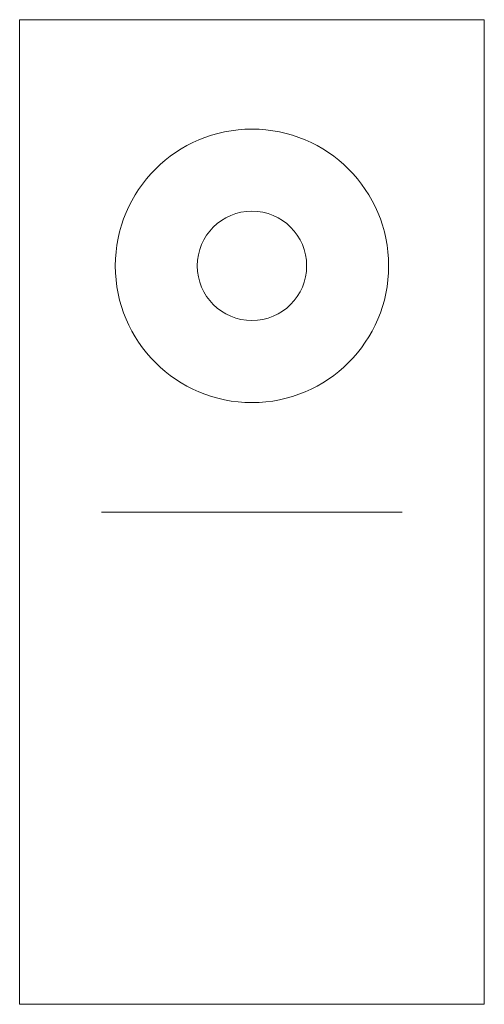
# Model space of a CAD drawing. Units: millimetres. Extents: x 2260 to 2345, y 1430 to 1610.
import ezdxf

# ---------------------------------------------------------------- set-up
doc = ezdxf.new("R2010")
doc.units = ezdxf.units.MM
doc.layers.add('M-CONS', color=8, linetype='Continuous', lineweight=13)

msp = doc.modelspace()

# ---------------------------------------------------------------- linework, layer by layer
at = {"layer": 'M-CONS', "extrusion": (-1, 0, 0)}
for p, q in [((2260.33, 1519.91), (2260.33, 1429.91)), ((2260.33, 1519.91, 25), (2260.33, 1429.91, 25))]:
    msp.add_line(p, q, dxfattribs=at)
at = {"layer": 'M-CONS'}
msp.add_line((2330.33, 1519.91, 25), (2275.33, 1519.91, 25), dxfattribs=at)
msp.add_lwpolyline([(2260.33, 1609.91), (2345.33, 1609.91), (2345.33, 1429.91), (2260.33, 1429.91)], close=True, dxfattribs=at)
at = {"layer": 'M-CONS', "extrusion": (-1, 0, 0), "elevation": -2260.33}
msp.add_lwpolyline([(-1519.91, 25), (-1495.42, 79.26, -0.645751), (-1454.4, 79.26), (-1429.91, 25)], format="xyb", close=True, dxfattribs=at)
at = {"layer": 'M-CONS', "extrusion": (0, 1, 0), "elevation": 1429.91}
msp.add_lwpolyline([(-2325.33, 0), (-2280.33, 0), (-2280.33, -10), (-2325.33, -10)], close=True, dxfattribs=at)
at = {"layer": 'M-CONS'}
for radius in [25, 10]:
    msp.add_circle((2302.83, 1564.91), radius, dxfattribs=at)
at = {"layer": 'M-CONS', "extrusion": (-1, 0, 0)}
msp.add_circle((-1474.91, 70, -2260.33), 15, dxfattribs=at)

doc.saveas('drawing.dxf')
